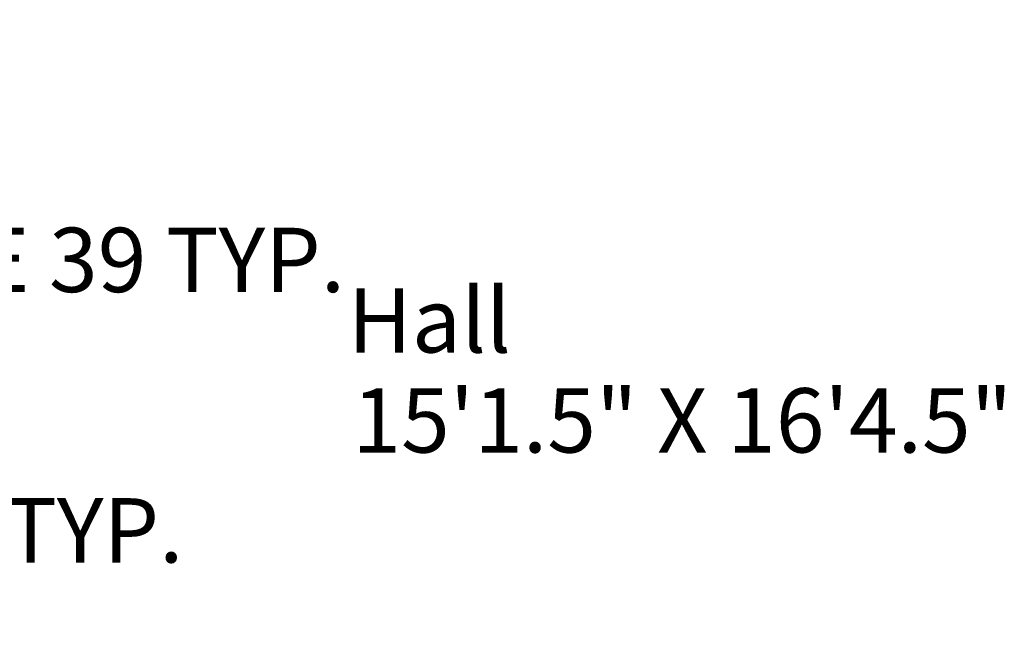
# Model space of a CAD drawing. Units: inches. Extents: x -1198 to -69, y -512 to 437.
# Tile 19 of 50: x -867 to -775, y 30 to 86. Entities that reach past the tile are written whole.
import ezdxf

# ---------------------------------------------------------------- set-up
doc = ezdxf.new("R2010")
doc.units = ezdxf.units.IN
doc.header["$MEASUREMENT"] = 0
doc.layers.add('A-ANNO-DIMS', color=2, linetype='Continuous', lineweight=18)
doc.layers.add('A-AREA-IDEN', color=7, linetype='Continuous', lineweight=18)
doc.styles.get("Standard").update_dxf_attribs({"font": 'arial.ttf'})
doc.dimstyles.get("Standard").update_dxf_attribs({"dimtxt": 6, "dimasz": 6, "dimexe": 0.18, "dimexo": 0.0625, "dimgap": 0.09, "dimtad": 0, "dimtih": 1, "dimtoh": 1, "dimdec": 0, "dimzin": 0, "dimdsep": 46, "dimlunit": 4, "dimtxsty": 'Standard', "dimblk": 'OBLIQUE', "dimcen": 0.09, "dimadec": 0, "dimazin": 0, "dimtfac": 1, "dimtdec": 0, "dimtofl": 0, "dimtmove": 0, "dimatfit": 3, "dimfxl": 1, "dimtolj": 1, "dimtzin": 0, "dimarcsym": 0})

# ---------------------------------------------------------------- blocks, each defined once
blk = doc.blocks.new('_Oblique')
at = {"color": 0, "linetype": 'ByBlock', "lineweight": -2}
blk.add_line((-0.5, -0.5), (0.5, 0.5), dxfattribs=at)
blk = doc.blocks.new('*D58')
at = {"layer": 'A-ANNO-DIMS', "color": 0, "lineweight": -2, "ltscale": 10, "transparency": 16777216}
for p, q in [((-881.718, 83.376), (-875.781, 83.376)), ((-875.961, 83.376), (-875.961, 67.177)), ((-875.961, 44.584), (-875.961, 60.784)), ((-881.718, 44.584), (-875.781, 44.584))]:
    blk.add_line(p, q, dxfattribs=at)
at = {"layer": 'DEFPOINTS', "color": 0, "ltscale": 10, "transparency": 16777216}
for p in [(-881.78, 83.376), (-875.961, 83.376), (-881.78, 44.584)]:
    blk.add_point(p, dxfattribs=at)
at = {"layer": 'A-ANNO-DIMS', "color": 0, "lineweight": -2, "ltscale": 10, "transparency": 16777216, "xscale": 6, "yscale": 6, "zscale": 6}
for p, rotation in [((-875.961, 83.376), 90), ((-875.961, 44.584), 270)]:
    blk.add_blockref('_Oblique', p, dxfattribs=dict(at, rotation=rotation))
at = {"layer": 'A-ANNO-DIMS', "color": 0, "ltscale": 10, "transparency": 16777216, "insert": (-875.961, 63.98), "char_height": 6, "attachment_point": 5}
blk.add_mtext('\\A1;TV CONSOLE 39 TYP.', dxfattribs=at)
blk = doc.blocks.new('*D59')
at = {"layer": 'A-ANNO-DIMS', "color": 0, "lineweight": -2, "ltscale": 10, "transparency": 16777216}
for p, q in [((-886.751, 44.522), (-886.751, 38.585)), ((-881.78, 44.522), (-881.78, 38.585)), ((-886.751, 38.765), (-881.78, 38.765)), ((-881.78, 38.765), (-875.78, 38.765))]:
    blk.add_line(p, q, dxfattribs=at)
at = {"layer": 'DEFPOINTS', "color": 0, "ltscale": 10, "transparency": 16777216}
for p in [(-886.751, 44.584), (-881.78, 44.584), (-881.78, 38.765)]:
    blk.add_point(p, dxfattribs=at)
at = {"layer": 'A-ANNO-DIMS', "color": 0, "lineweight": -2, "ltscale": 10, "transparency": 16777216, "xscale": 6, "yscale": 6, "zscale": 6, "rotation": 180}
blk.add_blockref('_Oblique', (-886.751, 38.765), dxfattribs=at)
at = {"layer": 'A-ANNO-DIMS', "color": 0, "lineweight": -2, "ltscale": 10, "transparency": 16777216, "xscale": 6, "yscale": 6, "zscale": 6}
blk.add_blockref('_Oblique', (-881.78, 38.765), dxfattribs=at)
at = {"layer": 'A-ANNO-DIMS', "color": 0, "ltscale": 10, "transparency": 16777216, "insert": (-863.418, 38.765), "char_height": 6, "attachment_point": 5}
blk.add_mtext('\\A1;5 TYP.', dxfattribs=at)

msp = doc.modelspace()

# ---------------------------------------------------------------- texts
at = {"layer": 'A-AREA-IDEN', "ltscale": 10, "char_height": 6, "attachment_point": 1}
for s, width, insert in [('Hall', 57.976527, (-836.5351, 61.3442)), ('15\'1.5" X 16\'4.5"', 62.175425, (-836.1157, 52.0171))]:
    msp.add_mtext_dynamic_manual_height_columns(s, width=width, gutter_width=30, heights=[0], dxfattribs=dict(at, insert=insert))

# ---------------------------------------------------------------- dimensions: what is measured, and where the dimension line sits
at = {"layer": 'A-ANNO-DIMS', "ltscale": 10}
dim = msp.add_linear_dim(base=(-875.9612, 83.3761), p1=(-881.78, 44.5842), p2=(-881.78, 83.3761), angle=90, text='TV CONSOLE <> TYP.', dimstyle='Standard', override={"dimdec": 0, "dimlfac": 1, "dimrnd": 0, "dimzin": 0, "dimdsep": 46, "dimlunit": 2}, dxfattribs=at)
dim.commit()
dim.dimension.update_dxf_attribs({"geometry": '*D58', "text_midpoint": (-875.9612, 63.9802)})
dim = msp.add_linear_dim(base=(-881.78, 38.7654), p1=(-886.7509, 44.5842), p2=(-881.78, 44.5842), text='<> TYP.', dimstyle='Standard', override={"dimdec": 0, "dimlfac": 1, "dimrnd": 0, "dimzin": 0, "dimdsep": 46, "dimlunit": 2}, dxfattribs=at)
dim.commit()
dim.dimension.update_dxf_attribs({"geometry": '*D59', "text_midpoint": (-863.4178, 38.7654)})

doc.saveas('drawing.dxf')
